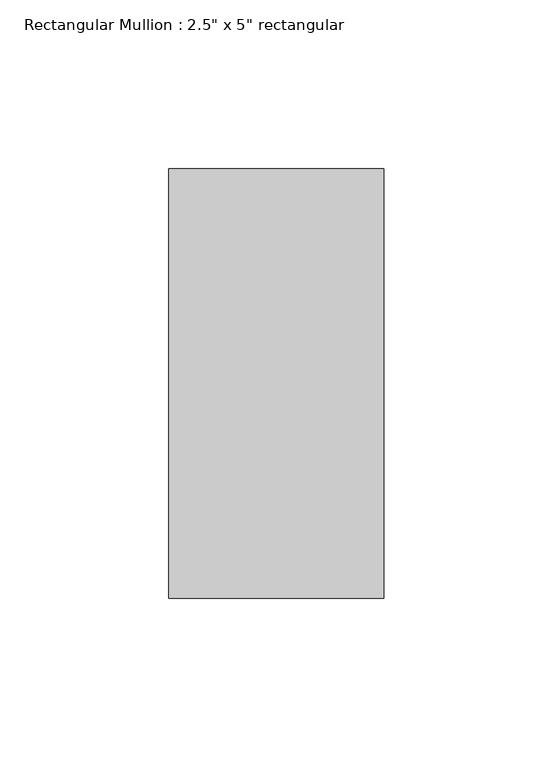
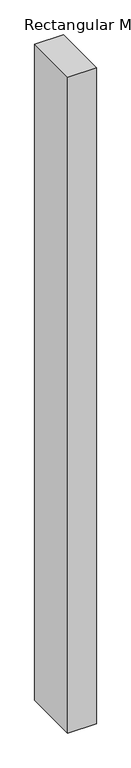
"""IFC4 building model written with IfcOpenShell, lengths in millimetres: member geometry."""

from ifc_helpers import new_model, si_unit, frame, origin, place, context, project, spatial, polyline, outline, extrude, source, transform, mapped, element, save


def member_78a9872f(model_context):
    return source(origin(), model_context, "Body", "SweptSolid", [
        extrude(outline(polyline([(31.75, 63.5), (31.75, -63.5), (-31.75, -63.5), (-31.75, 63.5), (31.75, 63.5)])), frame((0.0, 0.0, -1538.1940157), z_axis=(0.0, 0.0, 1.0), x_axis=(1.0, 0.0, 0.0)), (0.0, 0.0, 1.0), 1538.1940157),
    ])


if __name__ == "__main__":
    model = new_model("IFC4")
    model_context = context("Model", 3, world=origin())
    ifc_project = project(units=[si_unit("LENGTHUNIT", "METRE", prefix="MILLI")], contexts=[model_context])
    site = spatial("IfcSite", under=ifc_project)
    building = spatial("IfcBuilding", under=site)
    placement = place(None, origin())
    member_shape = member_78a9872f(model_context)
    element("IfcMember", 1, ObjectType="Rectangular Mullion : 2.5\" x 5\" rectangular", at=placement, inside=building, context=model_context, shape_type="MappedRepresentation", body=[
        mapped(member_shape, transform((0.0, 0.0, 0.0), x_axis=(1.0, 0.0, 0.0), y_axis=(0.0, 1.0, 0.0), z_axis=(0.0, 0.0, 1.0))),
    ])
    save(model, "model.ifc")

# Revit data of these elements
# Type "Rectangular Mullion : 2.5\" x 5\" rectangular"
#   built-in parameter 1007304 = 0.416667 (stored number, unit not read)
#   built-in parameter 1007301 = 0.104167 (stored number, unit not read)
#   built-in parameter 1007300 = 0.104167 (stored number, unit not read)
# Element 1 (IfcMember, "Rectangular Mullion : 2.5\" x 5\" rectangular")
#   Materials on its faces: "Aluminum"
# Materials
#   "Aluminum": class "Metal", colour RGB 247 247 247, transparency 0, Description = "Aluminum 6061", Cost = 0
